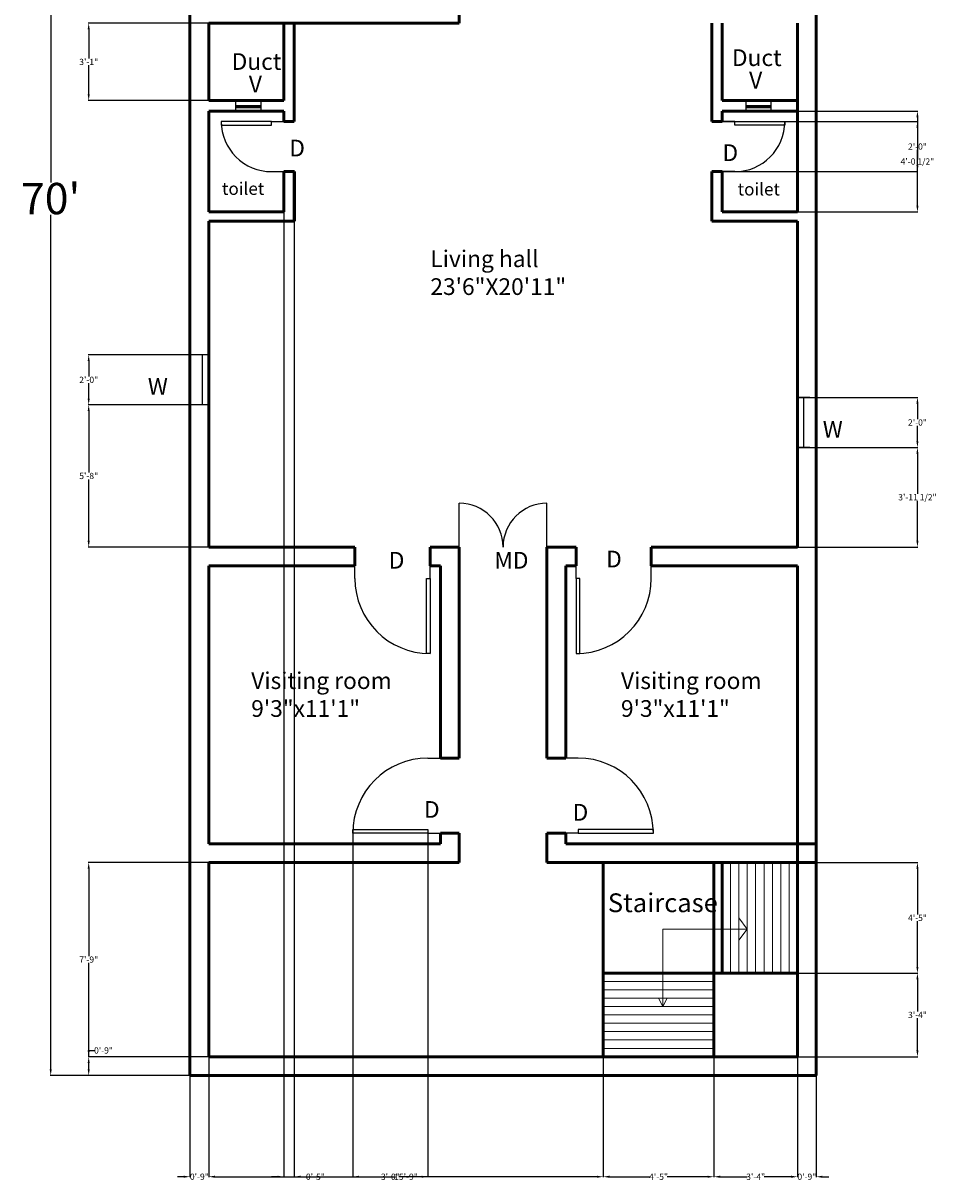
# Model space of a CAD drawing. Units: inches. Extents: x -250 to 2650, y 180 to 1183.
# Tile 5 of 10: x 952 to 1389, y 180 to 734. Entities that reach past the tile are written whole.
import ezdxf

# ---------------------------------------------------------------- set-up
doc = ezdxf.new("R2010")
doc.units = ezdxf.units.IN
doc.header["$MEASUREMENT"] = 0
for name, color, linetype, lineweight in [('A-ANNO-DIMS', 2, 'Continuous', 18), ('A-ANNO-TEXT', 7, 'Continuous', 18), ('A-AREA-IDEN', 3, 'Continuous', 18), ('A-DOOR', 4, 'Continuous', 25), ('A-FLOR-STRS', 8, 'Continuous', 18), ('A-GLAZ', 3, 'Continuous', 25), ('A-WALL', 7, 'Continuous', 50)]:
    doc.layers.add(name, color=color, linetype=linetype, lineweight=lineweight)
doc.styles.get("Standard").update_dxf_attribs({"font": 'arial.ttf'})
doc.dimstyles.get("Standard").update_dxf_attribs({"dimtxt": 3, "dimasz": 3, "dimexe": 0.18, "dimexo": 0.0625, "dimgap": 0.09, "dimtad": 0, "dimtih": 1, "dimtoh": 1, "dimdec": 0, "dimzin": 0, "dimdsep": 46, "dimlunit": 3, "dimtxsty": 'Standard', "dimcen": 0.09, "dimadec": 0, "dimazin": 0, "dimtfac": 1, "dimtdec": 0, "dimtofl": 0, "dimtmove": 0, "dimatfit": 3, "dimfxl": 1, "dimtolj": 1, "dimtzin": 0, "dimarcsym": 0})

# ---------------------------------------------------------------- blocks, each defined once
blk = doc.blocks.new('*D35')
at = {"layer": 'A-ANNO-DIMS', "color": 0, "lineweight": -2, "transparency": 16777216}
for p, q in [((1031.65, 1070.02), (964.83, 1070.02)), ((965.01, 1067.02), (965.01, 657.77)), ((965.01, 233.02), (965.01, 642.28)), ((1031.65, 230.02), (964.83, 230.02))]:
    blk.add_line(p, q, dxfattribs=at)
at = {"layer": 'A-ANNO-DIMS', "color": 0, "transparency": 16777216}
for points in [[(964.51, 1067.02), (965.51, 1067.02), (965.01, 1070.02)], [(964.51, 233.02), (965.51, 233.02), (965.01, 230.02)]]:
    blk.add_solid(points, dxfattribs=at)
at = {"layer": 'Defpoints', "color": 0, "transparency": 16777216}
for p in [(1031.71, 1070.02), (965.01, 230.02), (1031.71, 230.02)]:
    blk.add_point(p, dxfattribs=at)
at = {"layer": 'A-ANNO-DIMS', "color": 0, "transparency": 16777216, "insert": (965.01, 650.02), "char_height": 3, "attachment_point": 5}
blk.add_mtext("\\A1;{\\H5x;70'}", dxfattribs=at)
blk = doc.blocks.new('*U27')
for p, q in [((0, 0), (0, -6)), ((24, 0), (24, -6))]:
    blk.add_line(p, q)
blk.add_lwpolyline([(0, 0), (0, 24), (1.75, 24), (1.75, 0)], close=True)
blk.add_arc((0, 0), 24, 0, 90)
blk = doc.blocks.new('*U28')
for p, q in [((0, 0), (0, 6)), ((24, 0), (24, 6))]:
    blk.add_line(p, q)
blk.add_lwpolyline([(0, 0), (0, -24), (1.75, -24), (1.75, 0)], close=True)
blk.add_arc((0, 0), 24, 270, 0)
blk = doc.blocks.new('*U29')
for p, q in [((0, 5), (0, 0)), ((0, 2.5), (12, 2.5)), ((12, 5), (12, 0))]:
    blk.add_line(p, q)
blk = doc.blocks.new('*U30')
for p, q in [((-36, 0), (-36, -6)), ((0, 0), (0, -6))]:
    blk.add_line(p, q)
blk.add_lwpolyline([(0, 0), (0, 36), (-1.75, 36), (-1.75, 0)], close=True)
blk.add_arc((0, 0), 36, 90, 180)
blk = doc.blocks.new('*U31')
for p, q in [((-36, 0), (-36, 6)), ((0, 0), (0, 6))]:
    blk.add_line(p, q)
blk.add_lwpolyline([(0, 0), (0, -36), (-1.75, -36), (-1.75, 0)], close=True)
blk.add_arc((0, 0), 36, 180, 270)
blk = doc.blocks.new('*U32')
for p, q in [((0, 0), (0, -6)), ((36, 0), (36, -6))]:
    blk.add_line(p, q)
blk.add_lwpolyline([(0, 0), (0, 36), (1.75, 36), (1.75, 0)], close=True)
blk.add_arc((0, 0), 36, 0, 90)
blk = doc.blocks.new('*U33')
for p, q in [((-36, 0), (-36, -6)), ((0, 0), (0, -6))]:
    blk.add_line(p, q)
blk.add_lwpolyline([(0, 0), (0, 36), (-1.75, 36), (-1.75, 0)], close=True)
blk.add_arc((0, 0), 36, 90, 180)
blk = doc.blocks.new('*U23')
for p, q in [((-24, 6), (-24, 0)), ((0, 6), (0, 0)), ((0, 3), (-24, 3))]:
    blk.add_line(p, q)
blk = doc.blocks.new('*U24')
for p, q in [((-24, 6), (-24, 0)), ((0, 6), (0, 0)), ((0, 3), (-24, 3))]:
    blk.add_line(p, q)
blk = doc.blocks.new('DOOR-DOUBLE-MAIN')
for p, q in [((505.08, 483.11), (505.08, 504.11)), ((505.08, 483.11), (505.08, 504.11)), ((547.08, 483.11), (547.08, 504.11))]:
    blk.add_line(p, q)
for centre, start, end in [((505.08, 483.11), 0, 90), ((505.08, 483.11), 0, 90), ((547.08, 483.11), 90, 180)]:
    blk.add_arc(centre, 21, start, end)
blk = doc.blocks.new('*D103')
at = {"layer": 'A-ANNO-DIMS', "color": 0, "lineweight": -2, "transparency": 16777216}
for p, q in [((1322.713776, 238.962048), (1322.713776, 181.344548)), ((1331.713776, 229.962048), (1331.713776, 181.344548)), ((1319.713776, 181.524548), (1316.713776, 181.524548)), ((1334.713776, 181.524548), (1337.713776, 181.524548))]:
    blk.add_line(p, q, dxfattribs=at)
at = {"layer": 'A-ANNO-DIMS', "color": 0, "transparency": 16777216}
for points in [[(1319.713776, 182.024548), (1319.713776, 181.024548), (1322.713776, 181.524548)], [(1334.713776, 182.024548), (1334.713776, 181.024548), (1331.713776, 181.524548)]]:
    blk.add_solid(points, dxfattribs=at)
at = {"layer": 'Defpoints', "color": 0, "transparency": 16777216}
for p in [(1322.713776, 239.024548), (1331.713776, 230.024548), (1331.713776, 181.524548)]:
    blk.add_point(p, dxfattribs=at)
at = {"layer": 'A-ANNO-DIMS', "color": 0, "transparency": 16777216, "insert": (1327.213776, 181.524548), "char_height": 3, "attachment_point": 5}
blk.add_mtext('\\A1;0\'-9"', dxfattribs=at)
blk = doc.blocks.new('*D104')
at = {"layer": 'A-ANNO-DIMS', "color": 0, "lineweight": -2, "transparency": 16777216}
for p, q in [((1040.713776, 238.962048), (1040.713776, 181.344548)), ((1031.713776, 229.962048), (1031.713776, 181.344548)), ((1028.713776, 181.524548), (1025.713776, 181.524548)), ((1043.713776, 181.524548), (1046.713776, 181.524548))]:
    blk.add_line(p, q, dxfattribs=at)
at = {"layer": 'A-ANNO-DIMS', "color": 0, "transparency": 16777216}
for points in [[(1028.713776, 182.024548), (1028.713776, 181.024548), (1031.713776, 181.524548)], [(1043.713776, 182.024548), (1043.713776, 181.024548), (1040.713776, 181.524548)]]:
    blk.add_solid(points, dxfattribs=at)
at = {"layer": 'Defpoints', "color": 0, "transparency": 16777216}
for p in [(1040.713776, 239.024548), (1031.713776, 230.024548), (1040.713776, 181.524548)]:
    blk.add_point(p, dxfattribs=at)
at = {"layer": 'A-ANNO-DIMS', "color": 0, "transparency": 16777216, "insert": (1036.213776, 181.524548), "char_height": 3, "attachment_point": 5}
blk.add_mtext('\\A1;0\'-9"', dxfattribs=at)
blk = doc.blocks.new('*D105')
at = {"layer": 'A-ANNO-DIMS', "color": 0, "lineweight": -2, "transparency": 16777216}
for p, q in [((1040.71, 238.96), (1040.71, 181.34)), ((1229.71, 238.96), (1229.71, 181.34)), ((1043.71, 181.52), (1130.11, 181.52)), ((1226.71, 181.52), (1140.32, 181.52))]:
    blk.add_line(p, q, dxfattribs=at)
at = {"layer": 'A-ANNO-DIMS', "color": 0, "transparency": 16777216}
for points in [[(1043.71, 182.02), (1043.71, 181.02), (1040.71, 181.52)], [(1226.71, 182.02), (1226.71, 181.02), (1229.71, 181.52)]]:
    blk.add_solid(points, dxfattribs=at)
at = {"layer": 'Defpoints', "color": 0, "transparency": 16777216}
for p in [(1040.71, 239.02), (1229.71, 239.02), (1229.71, 181.52)]:
    blk.add_point(p, dxfattribs=at)
at = {"layer": 'A-ANNO-DIMS', "color": 0, "transparency": 16777216, "insert": (1135.21, 181.52), "char_height": 3, "attachment_point": 5}
blk.add_mtext('\\A1;15\'-9"', dxfattribs=at)
blk = doc.blocks.new('*D106')
at = {"layer": 'A-ANNO-DIMS', "color": 0, "lineweight": -2, "transparency": 16777216}
for p, q in [((1229.71, 238.96), (1229.71, 181.34)), ((1282.71, 238.96), (1282.71, 181.34)), ((1232.71, 181.52), (1252.08, 181.52)), ((1279.71, 181.52), (1260.35, 181.52))]:
    blk.add_line(p, q, dxfattribs=at)
at = {"layer": 'A-ANNO-DIMS', "color": 0, "transparency": 16777216}
for points in [[(1232.71, 182.02), (1232.71, 181.02), (1229.71, 181.52)], [(1279.71, 182.02), (1279.71, 181.02), (1282.71, 181.52)]]:
    blk.add_solid(points, dxfattribs=at)
at = {"layer": 'Defpoints', "color": 0, "transparency": 16777216}
for p in [(1229.71, 239.02), (1282.71, 239.02), (1282.71, 181.52)]:
    blk.add_point(p, dxfattribs=at)
at = {"layer": 'A-ANNO-DIMS', "color": 0, "transparency": 16777216, "insert": (1256.21, 181.52), "char_height": 3, "attachment_point": 5}
blk.add_mtext('\\A1;4\'-5"', dxfattribs=at)
blk = doc.blocks.new('*D107')
at = {"layer": 'A-ANNO-DIMS', "color": 0, "lineweight": -2, "transparency": 16777216}
for p, q in [((1282.71, 238.96), (1282.71, 181.34)), ((1322.71, 238.96), (1322.71, 181.34)), ((1285.71, 181.52), (1298.64, 181.52)), ((1319.71, 181.52), (1306.79, 181.52))]:
    blk.add_line(p, q, dxfattribs=at)
at = {"layer": 'A-ANNO-DIMS', "color": 0, "transparency": 16777216}
for points in [[(1285.71, 182.02), (1285.71, 181.02), (1282.71, 181.52)], [(1319.71, 182.02), (1319.71, 181.02), (1322.71, 181.52)]]:
    blk.add_solid(points, dxfattribs=at)
at = {"layer": 'Defpoints', "color": 0, "transparency": 16777216}
for p in [(1282.71, 239.02), (1322.71, 239.02), (1322.71, 181.52)]:
    blk.add_point(p, dxfattribs=at)
at = {"layer": 'A-ANNO-DIMS', "color": 0, "transparency": 16777216, "insert": (1302.71, 181.52), "char_height": 3, "attachment_point": 5}
blk.add_mtext('\\A1;3\'-4"', dxfattribs=at)
blk = doc.blocks.new('*D108')
at = {"layer": 'A-ANNO-DIMS', "color": 0, "lineweight": -2, "transparency": 16777216}
for p, q in [((1322.78, 279.02), (1380.39, 279.02)), ((1380.21, 276.02), (1380.21, 260.65)), ((1380.21, 242.02), (1380.21, 257.4)), ((1322.78, 239.02), (1380.39, 239.02))]:
    blk.add_line(p, q, dxfattribs=at)
at = {"layer": 'A-ANNO-DIMS', "color": 0, "transparency": 16777216}
for points in [[(1379.71, 276.02), (1380.71, 276.02), (1380.21, 279.02)], [(1379.71, 242.02), (1380.71, 242.02), (1380.21, 239.02)]]:
    blk.add_solid(points, dxfattribs=at)
at = {"layer": 'Defpoints', "color": 0, "transparency": 16777216}
for p in [(1322.71, 279.02), (1380.21, 279.02), (1322.71, 239.02)]:
    blk.add_point(p, dxfattribs=at)
at = {"layer": 'A-ANNO-DIMS', "color": 0, "transparency": 16777216, "insert": (1380.21, 259.02), "char_height": 3, "attachment_point": 5}
blk.add_mtext('\\A1;3\'-4"', dxfattribs=at)
blk = doc.blocks.new('*D109')
at = {"layer": 'A-ANNO-DIMS', "color": 0, "lineweight": -2, "transparency": 16777216}
for p, q in [((1318.78, 332.02), (1380.39, 332.02)), ((1380.21, 329.02), (1380.21, 307.14)), ((1380.21, 282.02), (1380.21, 303.91)), ((1322.78, 279.02), (1380.39, 279.02))]:
    blk.add_line(p, q, dxfattribs=at)
at = {"layer": 'A-ANNO-DIMS', "color": 0, "transparency": 16777216}
for points in [[(1379.71, 329.02), (1380.71, 329.02), (1380.21, 332.02)], [(1379.71, 282.02), (1380.71, 282.02), (1380.21, 279.02)]]:
    blk.add_solid(points, dxfattribs=at)
at = {"layer": 'Defpoints', "color": 0, "transparency": 16777216}
for p in [(1318.71, 332.02), (1380.21, 332.02), (1322.71, 279.02)]:
    blk.add_point(p, dxfattribs=at)
at = {"layer": 'A-ANNO-DIMS', "color": 0, "transparency": 16777216, "insert": (1380.21, 305.52), "char_height": 3, "attachment_point": 5}
blk.add_mtext('\\A1;4\'-5"', dxfattribs=at)
blk = doc.blocks.new('*D110')
at = {"layer": 'A-ANNO-DIMS', "color": 0, "lineweight": -2, "transparency": 16777216}
for p, q in [((1040.65, 239.02), (983.03, 239.02)), ((983.21, 239.02), (983.21, 242.02)), ((983.21, 242.02), (986.21, 242.02)), ((983.21, 233.02), (983.21, 236.02)), ((1031.65, 230.02), (983.03, 230.02))]:
    blk.add_line(p, q, dxfattribs=at)
at = {"layer": 'A-ANNO-DIMS', "color": 0, "transparency": 16777216}
for points in [[(982.71, 236.02), (983.71, 236.02), (983.21, 239.02)], [(982.71, 233.02), (983.71, 233.02), (983.21, 230.02)]]:
    blk.add_solid(points, dxfattribs=at)
at = {"layer": 'Defpoints', "color": 0, "transparency": 16777216}
for p in [(983.21, 239.02), (1040.71, 239.02), (1031.71, 230.02)]:
    blk.add_point(p, dxfattribs=at)
at = {"layer": 'A-ANNO-DIMS', "color": 0, "transparency": 16777216, "insert": (990.29, 242.02), "char_height": 3, "attachment_point": 5}
blk.add_mtext('\\A1;0\'-9"', dxfattribs=at)
blk = doc.blocks.new('*D111')
at = {"layer": 'A-ANNO-DIMS', "color": 0, "lineweight": -2, "transparency": 16777216}
for p, q in [((1040.65, 332.02), (983.03, 332.02)), ((983.21, 329.02), (983.21, 287.15)), ((983.21, 242.02), (983.21, 283.9)), ((1040.65, 239.02), (983.03, 239.02))]:
    blk.add_line(p, q, dxfattribs=at)
at = {"layer": 'A-ANNO-DIMS', "color": 0, "transparency": 16777216}
for points in [[(982.71, 329.02), (983.71, 329.02), (983.21, 332.02)], [(982.71, 242.02), (983.71, 242.02), (983.21, 239.02)]]:
    blk.add_solid(points, dxfattribs=at)
at = {"layer": 'Defpoints', "color": 0, "transparency": 16777216}
for p in [(983.21, 332.02), (1040.71, 332.02), (1040.71, 239.02)]:
    blk.add_point(p, dxfattribs=at)
at = {"layer": 'A-ANNO-DIMS', "color": 0, "transparency": 16777216, "insert": (983.21, 285.52), "char_height": 3, "attachment_point": 5}
blk.add_mtext('\\A1;7\'-9"', dxfattribs=at)
blk = doc.blocks.new('*D113')
at = {"layer": 'A-ANNO-DIMS', "color": 0, "lineweight": -2, "transparency": 16777216}
for p, q in [((1076.72, 643.56), (1076.72, 181.34)), ((1081.71, 639.05), (1081.71, 181.34)), ((1073.72, 181.52), (1070.72, 181.52)), ((1084.71, 181.52), (1087.71, 181.52))]:
    blk.add_line(p, q, dxfattribs=at)
at = {"layer": 'A-ANNO-DIMS', "color": 0, "transparency": 16777216}
for points in [[(1073.72, 182.02), (1073.72, 181.02), (1076.72, 181.52)], [(1084.71, 182.02), (1084.71, 181.02), (1081.71, 181.52)]]:
    blk.add_solid(points, dxfattribs=at)
at = {"layer": 'Defpoints', "color": 0, "transparency": 16777216}
for p in [(1076.72, 643.62), (1081.71, 639.11), (1081.71, 181.52)]:
    blk.add_point(p, dxfattribs=at)
at = {"layer": 'A-ANNO-DIMS', "color": 0, "transparency": 16777216, "insert": (1091.79, 181.52), "char_height": 3, "attachment_point": 5}
blk.add_mtext('\\A1;0\'-5"', dxfattribs=at)
blk = doc.blocks.new('*D114')
at = {"layer": 'A-ANNO-DIMS', "color": 0, "lineweight": -2, "transparency": 16777216}
for p, q in [((1040.65, 734.02), (983.03, 734.02)), ((983.21, 731.02), (983.21, 717.09)), ((983.21, 699.91), (983.21, 713.84)), ((1040.65, 696.91), (983.03, 696.91))]:
    blk.add_line(p, q, dxfattribs=at)
at = {"layer": 'A-ANNO-DIMS', "color": 0, "transparency": 16777216}
for points in [[(982.71, 731.02), (983.71, 731.02), (983.21, 734.02)], [(982.71, 699.91), (983.71, 699.91), (983.21, 696.91)]]:
    blk.add_solid(points, dxfattribs=at)
at = {"layer": 'Defpoints', "color": 0, "transparency": 16777216}
for p in [(983.21, 734.02), (1040.71, 734.02), (1040.71, 696.91)]:
    blk.add_point(p, dxfattribs=at)
at = {"layer": 'A-ANNO-DIMS', "color": 0, "transparency": 16777216, "insert": (983.21, 715.47), "char_height": 3, "attachment_point": 5}
blk.add_mtext('\\A1;3\'-1"', dxfattribs=at)
blk = doc.blocks.new('*D115')
at = {"layer": 'A-ANNO-DIMS', "color": 0, "lineweight": -2, "transparency": 16777216}
for p, q in [((1322.78, 691.91), (1380.39, 691.91)), ((1380.21, 688.91), (1380.21, 669.41)), ((1380.21, 646.62), (1380.21, 666.12)), ((1322.78, 643.62), (1380.39, 643.62))]:
    blk.add_line(p, q, dxfattribs=at)
at = {"layer": 'A-ANNO-DIMS', "color": 0, "transparency": 16777216}
for points in [[(1379.71, 688.91), (1380.71, 688.91), (1380.21, 691.91)], [(1379.71, 646.62), (1380.71, 646.62), (1380.21, 643.62)]]:
    blk.add_solid(points, dxfattribs=at)
at = {"layer": 'Defpoints', "color": 0, "transparency": 16777216}
for p in [(1322.71, 691.91), (1380.21, 691.91), (1322.71, 643.62)]:
    blk.add_point(p, dxfattribs=at)
at = {"layer": 'A-ANNO-DIMS', "color": 0, "transparency": 16777216, "insert": (1380.21, 667.77), "char_height": 3, "attachment_point": 5}
blk.add_mtext('\\A1;4\'-0 1/2"', dxfattribs=at)
blk = doc.blocks.new('*D116')
at = {"layer": 'A-ANNO-DIMS', "color": 0, "lineweight": -2, "transparency": 16777216}
for p, q in [((1322.78, 530.79), (1380.39, 530.79)), ((1380.21, 527.79), (1380.21, 508.59)), ((1380.21, 486.11), (1380.21, 505.31)), ((1322.78, 483.11), (1380.39, 483.11))]:
    blk.add_line(p, q, dxfattribs=at)
at = {"layer": 'A-ANNO-DIMS', "color": 0, "transparency": 16777216}
for points in [[(1379.71, 527.79), (1380.71, 527.79), (1380.21, 530.79)], [(1379.71, 486.11), (1380.71, 486.11), (1380.21, 483.11)]]:
    blk.add_solid(points, dxfattribs=at)
at = {"layer": 'Defpoints', "color": 0, "transparency": 16777216}
for p in [(1322.71, 530.79), (1380.21, 530.79), (1322.71, 483.11)]:
    blk.add_point(p, dxfattribs=at)
at = {"layer": 'A-ANNO-DIMS', "color": 0, "transparency": 16777216, "insert": (1380.21, 506.95), "char_height": 3, "attachment_point": 5}
blk.add_mtext('\\A1;3\'-11 1/2"', dxfattribs=at)
blk = doc.blocks.new('*D117')
at = {"layer": 'A-ANNO-DIMS', "color": 0, "lineweight": -2, "transparency": 16777216}
for p, q in [((1322.78, 554.79), (1380.39, 554.79)), ((1380.21, 551.79), (1380.21, 544.41)), ((1380.21, 533.79), (1380.21, 541.16)), ((1322.78, 530.79), (1380.39, 530.79))]:
    blk.add_line(p, q, dxfattribs=at)
at = {"layer": 'A-ANNO-DIMS', "color": 0, "transparency": 16777216}
for points in [[(1379.71, 551.79), (1380.71, 551.79), (1380.21, 554.79)], [(1379.71, 533.79), (1380.71, 533.79), (1380.21, 530.79)]]:
    blk.add_solid(points, dxfattribs=at)
at = {"layer": 'Defpoints', "color": 0, "transparency": 16777216}
for p in [(1322.71, 554.79), (1380.21, 554.79), (1322.71, 530.79)]:
    blk.add_point(p, dxfattribs=at)
at = {"layer": 'A-ANNO-DIMS', "color": 0, "transparency": 16777216, "insert": (1380.21, 542.79), "char_height": 3, "attachment_point": 5}
blk.add_mtext('\\A1;2\'-0"', dxfattribs=at)
blk = doc.blocks.new('*D118')
at = {"layer": 'A-ANNO-DIMS', "color": 0, "lineweight": -2, "transparency": 16777216}
for p, q in [((1040.65, 551.2), (983.03, 551.2)), ((983.21, 548.2), (983.21, 518.78)), ((983.21, 486.11), (983.21, 515.53)), ((1040.65, 483.11), (983.03, 483.11))]:
    blk.add_line(p, q, dxfattribs=at)
at = {"layer": 'A-ANNO-DIMS', "color": 0, "transparency": 16777216}
for points in [[(982.71, 548.2), (983.71, 548.2), (983.21, 551.2)], [(982.71, 486.11), (983.71, 486.11), (983.21, 483.11)]]:
    blk.add_solid(points, dxfattribs=at)
at = {"layer": 'Defpoints', "color": 0, "transparency": 16777216}
for p in [(983.21, 551.2), (1040.71, 551.2), (1040.71, 483.11)]:
    blk.add_point(p, dxfattribs=at)
at = {"layer": 'A-ANNO-DIMS', "color": 0, "transparency": 16777216, "insert": (983.21, 517.16), "char_height": 3, "attachment_point": 5}
blk.add_mtext('\\A1;5\'-8"', dxfattribs=at)
blk = doc.blocks.new('*D119')
at = {"layer": 'A-ANNO-DIMS', "color": 0, "lineweight": -2, "transparency": 16777216}
for p, q in [((1040.65, 575.2), (983.03, 575.2)), ((983.21, 572.2), (983.21, 564.82)), ((983.21, 554.2), (983.21, 561.58)), ((1040.65, 551.2), (983.03, 551.2))]:
    blk.add_line(p, q, dxfattribs=at)
at = {"layer": 'A-ANNO-DIMS', "color": 0, "transparency": 16777216}
for points in [[(982.71, 572.2), (983.71, 572.2), (983.21, 575.2)], [(982.71, 554.2), (983.71, 554.2), (983.21, 551.2)]]:
    blk.add_solid(points, dxfattribs=at)
at = {"layer": 'Defpoints', "color": 0, "transparency": 16777216}
for p in [(983.21, 575.2), (1040.71, 575.2), (1040.71, 551.2)]:
    blk.add_point(p, dxfattribs=at)
at = {"layer": 'A-ANNO-DIMS', "color": 0, "transparency": 16777216, "insert": (983.21, 563.2), "char_height": 3, "attachment_point": 5}
blk.add_mtext('\\A1;2\'-0"', dxfattribs=at)
blk = doc.blocks.new('*D120')
at = {"layer": 'A-ANNO-DIMS', "color": 0, "lineweight": -2, "transparency": 16777216}
for p, q in [((1109.71, 345.96), (1109.71, 181.34)), ((1145.71, 345.96), (1145.71, 181.34)), ((1112.71, 181.52), (1123.64, 181.52)), ((1142.71, 181.52), (1131.79, 181.52))]:
    blk.add_line(p, q, dxfattribs=at)
at = {"layer": 'A-ANNO-DIMS', "color": 0, "transparency": 16777216}
for points in [[(1112.71, 182.02), (1112.71, 181.02), (1109.71, 181.52)], [(1142.71, 182.02), (1142.71, 181.02), (1145.71, 181.52)]]:
    blk.add_solid(points, dxfattribs=at)
at = {"layer": 'Defpoints', "color": 0, "transparency": 16777216}
for p in [(1109.71, 346.02), (1145.71, 346.02), (1145.71, 181.52)]:
    blk.add_point(p, dxfattribs=at)
at = {"layer": 'A-ANNO-DIMS', "color": 0, "transparency": 16777216, "insert": (1127.71, 181.52), "char_height": 3, "attachment_point": 5}
blk.add_mtext('\\A1;3\'-0"', dxfattribs=at)
blk = doc.blocks.new('*D121')
at = {"layer": 'A-ANNO-DIMS', "color": 0, "lineweight": -2, "transparency": 16777216}
for p, q in [((1281.78, 686.91), (1380.39, 686.91)), ((1380.21, 683.91), (1380.21, 676.53)), ((1380.21, 665.91), (1380.21, 673.29)), ((1281.78, 662.91), (1380.39, 662.91))]:
    blk.add_line(p, q, dxfattribs=at)
at = {"layer": 'A-ANNO-DIMS', "color": 0, "transparency": 16777216}
for points in [[(1379.71, 683.91), (1380.71, 683.91), (1380.21, 686.91)], [(1379.71, 665.91), (1380.71, 665.91), (1380.21, 662.91)]]:
    blk.add_solid(points, dxfattribs=at)
at = {"layer": 'Defpoints', "color": 0, "transparency": 16777216}
for p in [(1281.71, 686.91), (1380.21, 686.91), (1281.71, 662.91)]:
    blk.add_point(p, dxfattribs=at)
at = {"layer": 'A-ANNO-DIMS', "color": 0, "transparency": 16777216, "insert": (1380.21, 674.91), "char_height": 3, "attachment_point": 5}
blk.add_mtext('\\A1;2\'-0"', dxfattribs=at)

msp = doc.modelspace()

# ---------------------------------------------------------------- linework, layer by layer
at = {"layer": 'A-FLOR-STRS'}
for p, q in [((1290.71, 279.02), (1290.71, 332.02)), ((1294.71, 279.02), (1294.71, 332.02)), ((1298.71, 279.02), (1298.71, 332.02)), ((1302.71, 279.02), (1302.71, 332.02)), ((1306.71, 279.02), (1306.71, 332.02)), ((1310.71, 279.02), (1310.71, 332.02)), ((1314.71, 279.02), (1314.71, 332.02)), ((1318.71, 279.02), (1318.71, 332.02)), ((1298.71, 300.14), (1294.71, 305.52)), ((1258.23, 300.14), (1258.23, 263.02)), ((1258.23, 300.14), (1298.71, 300.14)), ((1298.71, 300.14), (1294.71, 294.75)), ((1229.71, 275.02), (1282.71, 275.02)), ((1229.71, 271.02), (1282.71, 271.02)), ((1229.71, 267.02), (1282.71, 267.02)), ((1258.23, 263.02), (1256.21, 267.02)), ((1258.23, 263.02), (1260.24, 267.02)), ((1229.71, 263.02), (1282.71, 263.02)), ((1229.71, 259.02), (1282.71, 259.02)), ((1229.71, 255.02), (1282.71, 255.02)), ((1229.71, 251.02), (1282.71, 251.02)), ((1229.71, 247.02), (1282.71, 247.02)), ((1229.71, 243.02), (1282.71, 243.02))]:
    msp.add_line(p, q, dxfattribs=at)
at = {"layer": 'A-WALL'}
for p, q in [((1031.71, 1070.02), (1031.71, 230.02)), ((1331.71, 230.02), (1331.71, 1070.02)), ((1160.71, 748.02), (1160.71, 734.02)), ((1160.71, 734.02), (1040.71, 734.02)), ((1040.71, 734.02), (1040.71, 696.91)), ((1076.71, 696.91), (1076.71, 734.02)), ((1081.71, 686.91), (1081.71, 734.02)), ((1281.71, 686.91), (1281.71, 734.02)), ((1281.71, 686.91), (1281.71, 734.02)), ((1286.71, 696.91), (1286.71, 734.02)), ((1322.71, 643.62), (1322.71, 734.02)), ((1322.71, 696.91), (1322.71, 734.02)), ((1322.71, 716.02), (1322.71, 734.02)), ((1076.71, 696.91), (1040.71, 696.91)), ((1065.77, 693.93), (1053.77, 693.93)), ((1322.71, 696.91), (1286.71, 696.91)), ((1310.15, 693.93), (1298.15, 693.93)), ((1040.71, 691.91), (1040.71, 643.62)), ((1076.72, 691.91), (1040.71, 691.91)), ((1076.72, 691.91), (1076.72, 686.91)), ((1286.71, 686.91), (1286.71, 691.91)), ((1322.71, 691.91), (1286.71, 691.91)), ((1322.71, 643.62), (1322.71, 691.91)), ((1076.72, 686.91), (1081.71, 686.91)), ((1286.71, 686.91), (1281.71, 686.91)), ((1076.72, 662.91), (1076.72, 643.62)), ((1076.72, 662.91), (1081.72, 662.91)), ((1081.71, 639.11), (1081.71, 662.91)), ((1081.72, 662.91), (1081.72, 639.11)), ((1281.71, 639.11), (1281.71, 662.91)), ((1281.71, 643.62), (1281.71, 662.91)), ((1286.71, 662.91), (1281.71, 662.91)), ((1286.71, 643.62), (1286.71, 662.91)), ((1076.72, 643.62), (1040.71, 643.62)), ((1081.72, 643.62), (1081.71, 643.62)), ((1322.71, 643.62), (1286.71, 643.62)), ((1040.71, 639.11), (1040.71, 483.11)), ((1081.72, 639.11), (1040.71, 639.11)), ((1322.71, 639.11), (1281.71, 639.11)), ((1322.71, 483.11), (1322.71, 639.11)), ((1322.71, 587.02), (1322.71, 639.11)), ((1110.71, 483.11), (1040.71, 483.11)), ((1110.71, 474.11), (1110.71, 483.11)), ((1160.71, 483.11), (1146.71, 483.11)), ((1146.71, 474.11), (1146.71, 483.11)), ((1160.71, 483.11), (1160.71, 382.02)), ((1202.71, 382.02), (1202.71, 483.11)), ((1216.71, 483.11), (1202.71, 483.11)), ((1216.71, 474.11), (1216.71, 483.11)), ((1322.71, 483.11), (1252.71, 483.11)), ((1252.71, 474.11), (1252.71, 483.11)), ((1040.71, 474.11), (1040.71, 341.02)), ((1110.71, 474.11), (1040.71, 474.11)), ((1151.71, 474.11), (1146.71, 474.11)), ((1151.71, 474.11), (1151.71, 382.02)), ((1211.71, 382.02), (1211.71, 474.11)), ((1216.71, 474.11), (1211.71, 474.11)), ((1322.71, 474.11), (1252.71, 474.11)), ((1322.71, 239.02), (1322.71, 474.11)), ((1151.71, 382.02), (1160.71, 382.02)), ((1202.71, 382.02), (1211.71, 382.02)), ((1151.71, 346.02), (1151.71, 341.02)), ((1151.71, 346.02), (1160.71, 346.02)), ((1160.71, 346.02), (1160.71, 332.02)), ((1202.71, 332.02), (1202.71, 346.02)), ((1211.71, 346.02), (1202.71, 346.02)), ((1211.71, 341.02), (1211.71, 346.02)), ((1040.71, 341.02), (1151.71, 341.02)), ((1211.71, 341.02), (1331.71, 341.02)), ((1040.71, 332.02), (1160.71, 332.02)), ((1040.71, 332.02), (1040.71, 239.02)), ((1202.71, 332.02), (1331.71, 332.02)), ((1229.71, 239.02), (1229.71, 332.02)), ((1282.71, 239.02), (1282.71, 332.02)), ((1286.71, 279.02), (1286.71, 332.02)), ((1229.71, 279.02), (1322.71, 279.02)), ((1040.71, 239.02), (1065.46, 239.02)), ((1040.71, 239.02), (1322.71, 239.02)), ((1031.71, 230.02), (1064.71, 230.02)), ((1031.71, 230.02), (1331.71, 230.02))]:
    msp.add_line(p, q, dxfattribs=at)

# ---------------------------------------------------------------- block references
at = {"layer": 'A-DOOR'}
for name, p, rotation in [('*U28', (1070.72, 686.91), 270), ('*U27', (1292.71, 686.91), 270), ('*U32', (1146.71, 468.11), 180), ('*U33', (1216.71, 468.11), 180), ('*U31', (1145.71, 346.02), 270), ('*U30', (1217.71, 346.02), 270)]:
    msp.add_blockref(name, p, dxfattribs=dict(at, rotation=rotation))
msp.add_blockref('DOOR-DOUBLE-MAIN', (655.63, 0), dxfattribs=at)
at = {"layer": 'A-GLAZ'}
for name, p, rotation in [('*U29', (1065.77, 696.91), 180), ('*U29', (1310.15, 696.91), 180), ('*U23', (1034.71, 551.2), 270), ('*U24', (1322.71, 530.79), 270)]:
    msp.add_blockref(name, p, dxfattribs=dict(at, rotation=rotation))

# ---------------------------------------------------------------- texts
at = {"layer": 'A-ANNO-TEXT', "char_height": 8, "attachment_point": 1}
for s, insert in [('V', (1299.58, 710.71)), ('V', (1059.93, 708.86)), ('D', (1079.29, 678.19)), ('D', (1286.8, 675.98)), ('W', (1011.54, 564.02)), ('W', (1334.85, 543.51)), ('D', (1126.95, 480.78)), ('MD', (1177.52, 480.78)), ('D', (1231.07, 481.35)), ('D', (1143.82, 361.42)), ('D', (1215.02, 360.07))]:
    msp.add_mtext_dynamic_manual_height_columns(s, width=10.3916, gutter_width=1, heights=[0], dxfattribs=dict(at, insert=insert))
at = {"layer": 'A-AREA-IDEN', "attachment_point": 1}
for s, width, heights, insert, char_height in [('{\\H2.66667x;Duct} ', 7.71, [3.05], (1291.33, 721.49), 3), ('{\\H2.66667x;Duct} ', 7.71, [3.05], (1051.68, 719.65), 3), ('toilet', 19.3499, [0], (1047.06, 657.78), 6), ('toilet', 19.3499, [0], (1294.1, 657.5), 6), ('Living hall  \\P23\'6"X20\'11"', 123.5412, [0], (1146.87, 625.18), 8), ('Visiting room 9\'3"x11\'1"', 88.0689, [0], (1061.06, 423.12), 8), ('Visiting room 9\'3"x11\'1"', 88.0689, [0], (1238.19, 423.12), 8), ('Staircase  ', 87.4783, [0], (1231.89, 317.24), 9)]:
    msp.add_mtext_dynamic_manual_height_columns(s, width=width, gutter_width=1, heights=heights, dxfattribs=dict(at, insert=insert, char_height=char_height))

# ---------------------------------------------------------------- dimensions: what is measured, and where the dimension line sits
at = {"layer": 'A-ANNO-DIMS'}
dim = msp.add_linear_dim(base=(965.01, 230.02), p1=(1031.71, 1070.02), p2=(1031.71, 230.02), angle=90, text='{\\H5x;<>}', dimstyle='Standard', override={"dimclrd": 0, "dimclre": 0, "dimclrt": 0}, dxfattribs=at)
dim.commit()
dim.dimension.update_dxf_attribs({"geometry": '*D35', "text_midpoint": (965.01, 650.02)})
for base, p1, p2, picture, middle in [((983.21, 734.02), (1040.71, 696.91), (1040.71, 734.02), '*D114', (983.21, 715.47)), ((1380.21, 691.91), (1322.71, 643.62), (1322.71, 691.91), '*D115', (1380.21, 667.77)), ((1380.21, 686.91), (1281.71, 662.91), (1281.71, 686.91), '*D121', (1380.21, 674.91)), ((983.21, 575.2), (1040.71, 551.2), (1040.71, 575.2), '*D119', (983.21, 563.2)), ((1380.21, 554.79), (1322.71, 530.79), (1322.71, 554.79), '*D117', (1380.21, 542.79)), ((983.21, 551.2), (1040.71, 483.11), (1040.71, 551.2), '*D118', (983.21, 517.16)), ((1380.21, 530.79), (1322.71, 483.11), (1322.71, 530.79), '*D116', (1380.21, 506.95)), ((983.21, 332.02), (1040.71, 239.02), (1040.71, 332.02), '*D111', (983.21, 285.52)), ((1380.21, 332.02), (1322.71, 279.02), (1318.71, 332.02), '*D109', (1380.21, 305.52)), ((1380.21, 279.02), (1322.71, 239.02), (1322.71, 279.02), '*D108', (1380.21, 259.02)), ((983.21, 239.02), (1031.71, 230.02), (1040.71, 239.02), '*D110', (990.29, 242.02))]:
    dim = msp.add_linear_dim(base=base, p1=p1, p2=p2, angle=90, dimstyle='Standard', override={"dimdec": 1, "dimlfac": 1, "dimrnd": 0, "dimzin": 1, "dimdsep": 46, "dimlunit": 4, "dimfrac": 2}, dxfattribs=at)
    dim.commit()
    dim.dimension.update_dxf_attribs({"geometry": picture, "text_midpoint": middle})
for base, p1, p2, picture, middle in [((1081.71, 181.52), (1076.72, 643.62), (1081.71, 639.11), '*D113', (1091.79, 181.52)), ((1145.71, 181.52), (1109.71, 346.02), (1145.71, 346.02), '*D120', (1127.71, 181.52)), ((1040.71, 181.52), (1031.71, 230.02), (1040.71, 239.02), '*D104', (1036.21, 181.52)), ((1229.71, 181.52), (1040.71, 239.02), (1229.71, 239.02), '*D105', (1135.21, 181.52)), ((1282.71, 181.52), (1229.71, 239.02), (1282.71, 239.02), '*D106', (1256.21, 181.52)), ((1322.71, 181.52), (1282.71, 239.02), (1322.71, 239.02), '*D107', (1302.71, 181.52)), ((1331.71, 181.52), (1322.71, 239.02), (1331.71, 230.02), '*D103', (1327.21, 181.52))]:
    dim = msp.add_linear_dim(base=base, p1=p1, p2=p2, dimstyle='Standard', override={"dimdec": 1, "dimlfac": 1, "dimrnd": 0, "dimzin": 1, "dimdsep": 46, "dimlunit": 4, "dimfrac": 2}, dxfattribs=at)
    dim.commit()
    dim.dimension.update_dxf_attribs({"geometry": picture, "text_midpoint": middle})

doc.saveas('drawing.dxf')
